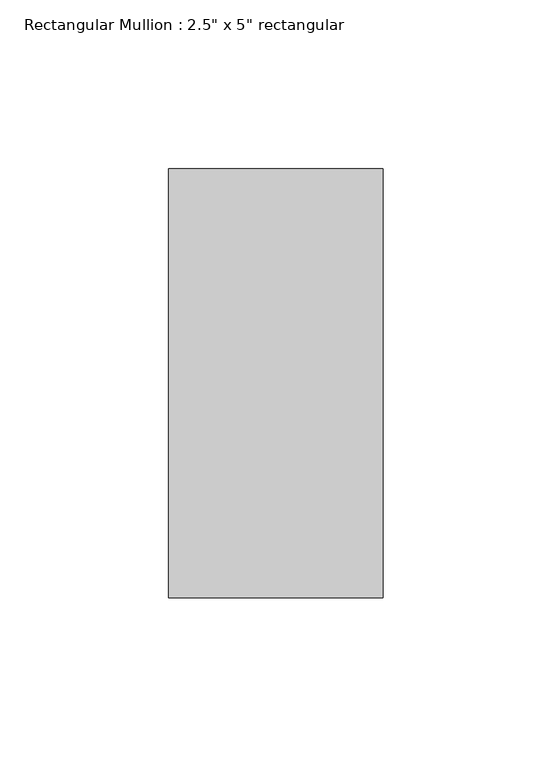
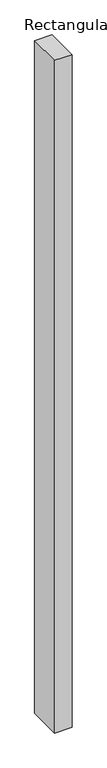
"""IFC4 building model written with IfcOpenShell, lengths in millimetres: member geometry."""

from ifc_helpers import new_model, si_unit, frame, origin, place, context, project, spatial, polyline, outline, extrude, source, transform, mapped, element, save


def member_70c1698b(model_context):
    return source(origin(), model_context, "Body", "SweptSolid", [
        extrude(outline(polyline([(0.0, 63.5), (0.0, -63.5), (-63.5, -63.5), (-63.5, 63.5), (0.0, 63.5)])), frame((0.0, 0.0, -2616.2), z_axis=(0.0, 0.0, 1.0), x_axis=(1.0, 0.0, 0.0)), (0.0, 0.0, 1.0), 2616.2),
    ])


if __name__ == "__main__":
    model = new_model("IFC4")
    model_context = context("Model", 3, world=origin())
    ifc_project = project(units=[si_unit("LENGTHUNIT", "METRE", prefix="MILLI")], contexts=[model_context])
    site = spatial("IfcSite", under=ifc_project)
    building = spatial("IfcBuilding", under=site)
    placement = place(None, origin())
    member_shape = member_70c1698b(model_context)
    element("IfcMember", 1, ObjectType="Rectangular Mullion : 2.5\" x 5\" rectangular", at=placement, inside=building, context=model_context, shape_type="MappedRepresentation", body=[
        mapped(member_shape, transform((0.0, 0.0, 0.0), x_axis=(1.0, 0.0, 0.0), y_axis=(0.0, 1.0, 0.0), z_axis=(0.0, 0.0, 1.0))),
    ])
    save(model, "model.ifc")

# Revit data of these elements
# Type "Rectangular Mullion : 2.5\" x 5\" rectangular"
#   built-in parameter 1007304 = 0.416667 (stored number, unit not read)
#   built-in parameter 1007301 = 0.104167 (stored number, unit not read)
#   built-in parameter 1007300 = 0.104167 (stored number, unit not read)
# Element 1 (IfcMember, "Rectangular Mullion : 2.5\" x 5\" rectangular")
#   Materials on its faces: "Iron, Ductile"
# Materials
#   "Iron, Ductile": class "Metal", colour RGB 0 0 0, transparency 0, Description = "Ductile cast iron", Cost = 0
